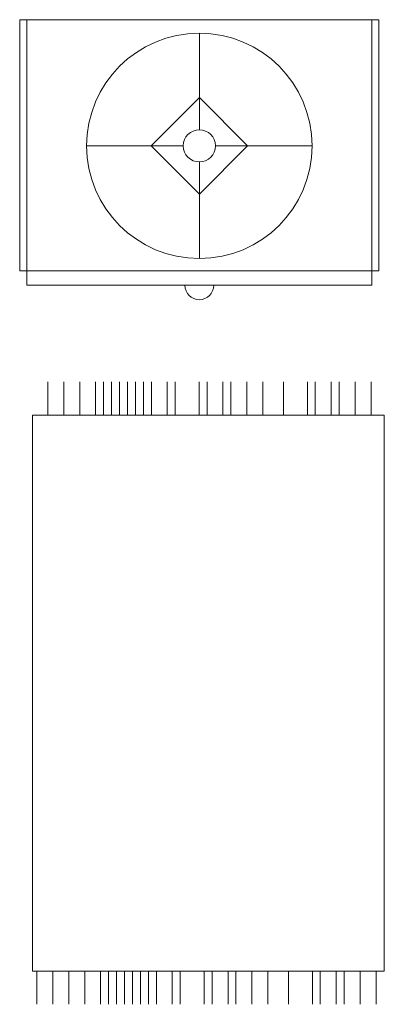
# Model space of a CAD drawing. Units: inches. Extents: x 1994 to 3075, y 3517 to 3950.
# Tile 17 of 58: x 1994.6593 to 1994.68726, y 3553.23973 to 3553.31519. Entities that reach past the tile are written whole.
import ezdxf

# ---------------------------------------------------------------- set-up
doc = ezdxf.new("R2010")
doc.units = ezdxf.units.IN
doc.layers.add('A-FURN-REFR', color=8, linetype='Continuous', lineweight=13)

msp = doc.modelspace()

# ---------------------------------------------------------------- linework, layer by layer
at = {"layer": 'A-FURN-REFR'}
for p, q in [((1994.659304, 3553.31519), (1994.659304, 3553.295937)), ((1994.686848, 3553.31519), (1994.659304, 3553.31519)), ((1994.659855, 3553.31519), (1994.659855, 3553.294835)), ((1994.686297, 3553.294835), (1994.686297, 3553.31519)), ((1994.686848, 3553.295937), (1994.686848, 3553.31519)), ((1994.673076, 3553.314159), (1994.673076, 3553.306755)), ((1994.673076, 3553.309223), (1994.669374, 3553.305521)), ((1994.676778, 3553.305521), (1994.673076, 3553.309223)), ((1994.671842, 3553.305521), (1994.664438, 3553.305521)), ((1994.669374, 3553.305521), (1994.673076, 3553.301819)), ((1994.673076, 3553.301819), (1994.676778, 3553.305521)), ((1994.67431, 3553.305521), (1994.681713, 3553.305521)), ((1994.673076, 3553.304287), (1994.673076, 3553.296884)), ((1994.659304, 3553.295937), (1994.686848, 3553.295937)), ((1994.659855, 3553.294835), (1994.686297, 3553.294835)), ((1994.661464, 3553.284896, -0.035802), (1994.661464, 3553.287437, -0.035802)), ((1994.662684, 3553.284896, -0.035802), (1994.662684, 3553.287437, -0.035802)), ((1994.663905, 3553.284896, -0.035802), (1994.663905, 3553.287437, -0.035802)), ((1994.665125, 3553.284896, -0.035802), (1994.665125, 3553.287437, -0.035802)), ((1994.665735, 3553.284896, -0.035802), (1994.665735, 3553.287437, -0.035802)), ((1994.666346, 3553.284896, -0.035802), (1994.666346, 3553.287437, -0.035802)), ((1994.666956, 3553.284896, -0.035802), (1994.666956, 3553.287437, -0.035802)), ((1994.667566, 3553.284896, -0.035802), (1994.667566, 3553.287437, -0.035802)), ((1994.668177, 3553.284896, -0.035802), (1994.668177, 3553.287437, -0.035802)), ((1994.668787, 3553.284896, -0.035802), (1994.668787, 3553.287437, -0.035802)), ((1994.669397, 3553.284896, -0.035802), (1994.669397, 3553.287437, -0.035802)), ((1994.670618, 3553.284896, -0.035802), (1994.670618, 3553.287437, -0.035802)), ((1994.671228, 3553.284896, -0.035802), (1994.671228, 3553.287437, -0.035802)), ((1994.673059, 3553.284896, -0.035802), (1994.673059, 3553.287437, -0.035802)), ((1994.673669, 3553.284896, -0.035802), (1994.673669, 3553.287437, -0.035802)), ((1994.674889, 3553.284896, -0.035802), (1994.674889, 3553.287437, -0.035802)), ((1994.6755, 3553.284896, -0.035802), (1994.6755, 3553.287437, -0.035802)), ((1994.67672, 3553.284896, -0.035802), (1994.67672, 3553.287437, -0.035802)), ((1994.67672, 3553.284896, -0.035802), (1994.67672, 3553.287437, -0.035802)), ((1994.677941, 3553.284896, -0.035802), (1994.677941, 3553.287437, -0.035802)), ((1994.679525, 3553.284896, -0.035802), (1994.679525, 3553.287437, -0.035802)), ((1994.681356, 3553.284896, -0.035802), (1994.681356, 3553.287437, -0.035802)), ((1994.681966, 3553.284896, -0.035802), (1994.681966, 3553.287437, -0.035802)), ((1994.683186, 3553.284896, -0.035802), (1994.683186, 3553.287437, -0.035802)), ((1994.683797, 3553.284896, -0.035802), (1994.683797, 3553.287437, -0.035802)), ((1994.685017, 3553.284896, -0.035802), (1994.685017, 3553.287437, -0.035802)), ((1994.685017, 3553.284896, -0.035802), (1994.685017, 3553.287437, -0.035802)), ((1994.686238, 3553.284896, -0.035802), (1994.686238, 3553.287437, -0.035802)), ((1994.660277, 3553.242273, -0.035802), (1994.660277, 3553.284894, -0.035802)), ((1994.687256, 3553.284894, -0.035802), (1994.660277, 3553.284894, -0.035802)), ((1994.687256, 3553.242273, -0.035802), (1994.687256, 3553.284894, -0.035802)), ((1994.687256, 3553.242273, -0.035802), (1994.660277, 3553.242273, -0.035802)), ((1994.660627, 3553.239733, -0.035802), (1994.660627, 3553.242273, -0.035802)), ((1994.661848, 3553.239733, -0.035802), (1994.661848, 3553.242273, -0.035802)), ((1994.663068, 3553.239733, -0.035802), (1994.663068, 3553.242273, -0.035802)), ((1994.664289, 3553.239733, -0.035802), (1994.664289, 3553.242273, -0.035802)), ((1994.665509, 3553.239733, -0.035802), (1994.665509, 3553.242273, -0.035802)), ((1994.66612, 3553.239733, -0.035802), (1994.66612, 3553.242273, -0.035802)), ((1994.66673, 3553.239733, -0.035802), (1994.66673, 3553.242273, -0.035802)), ((1994.66734, 3553.239733, -0.035802), (1994.66734, 3553.242273, -0.035802)), ((1994.66795, 3553.239733, -0.035802), (1994.66795, 3553.242273, -0.035802)), ((1994.668561, 3553.239733, -0.035802), (1994.668561, 3553.242273, -0.035802)), ((1994.669171, 3553.239733, -0.035802), (1994.669171, 3553.242273, -0.035802)), ((1994.669781, 3553.239733, -0.035802), (1994.669781, 3553.242273, -0.035802)), ((1994.671002, 3553.239733, -0.035802), (1994.671002, 3553.242273, -0.035802)), ((1994.671612, 3553.239733, -0.035802), (1994.671612, 3553.242273, -0.035802)), ((1994.673443, 3553.239733, -0.035802), (1994.673443, 3553.242273, -0.035802)), ((1994.674053, 3553.239733, -0.035802), (1994.674053, 3553.242273, -0.035802)), ((1994.675274, 3553.239733, -0.035802), (1994.675274, 3553.242273, -0.035802)), ((1994.675884, 3553.239733, -0.035802), (1994.675884, 3553.242273, -0.035802)), ((1994.677104, 3553.239733, -0.035802), (1994.677104, 3553.242273, -0.035802)), ((1994.677104, 3553.239733, -0.035802), (1994.677104, 3553.242273, -0.035802)), ((1994.678325, 3553.239733, -0.035802), (1994.678325, 3553.242273, -0.035802)), ((1994.679909, 3553.239733, -0.035802), (1994.679909, 3553.242273, -0.035802)), ((1994.68174, 3553.239733, -0.035802), (1994.68174, 3553.242273, -0.035802)), ((1994.68235, 3553.239733, -0.035802), (1994.68235, 3553.242273, -0.035802)), ((1994.68357, 3553.239733, -0.035802), (1994.68357, 3553.242273, -0.035802)), ((1994.684181, 3553.239733, -0.035802), (1994.684181, 3553.242273, -0.035802)), ((1994.685401, 3553.239733, -0.035802), (1994.685401, 3553.242273, -0.035802)), ((1994.685401, 3553.239733, -0.035802), (1994.685401, 3553.242273, -0.035802)), ((1994.686622, 3553.239733, -0.035802), (1994.686622, 3553.242273, -0.035802))]:
    msp.add_line(p, q, dxfattribs=at)
for radius in [0.008638, 0.001234]:
    msp.add_circle((1994.673076, 3553.305521), radius, dxfattribs=at)
msp.add_arc((1994.673076, 3553.294835), 0.001102, 180, 0, dxfattribs=at)

doc.saveas('drawing.dxf')
